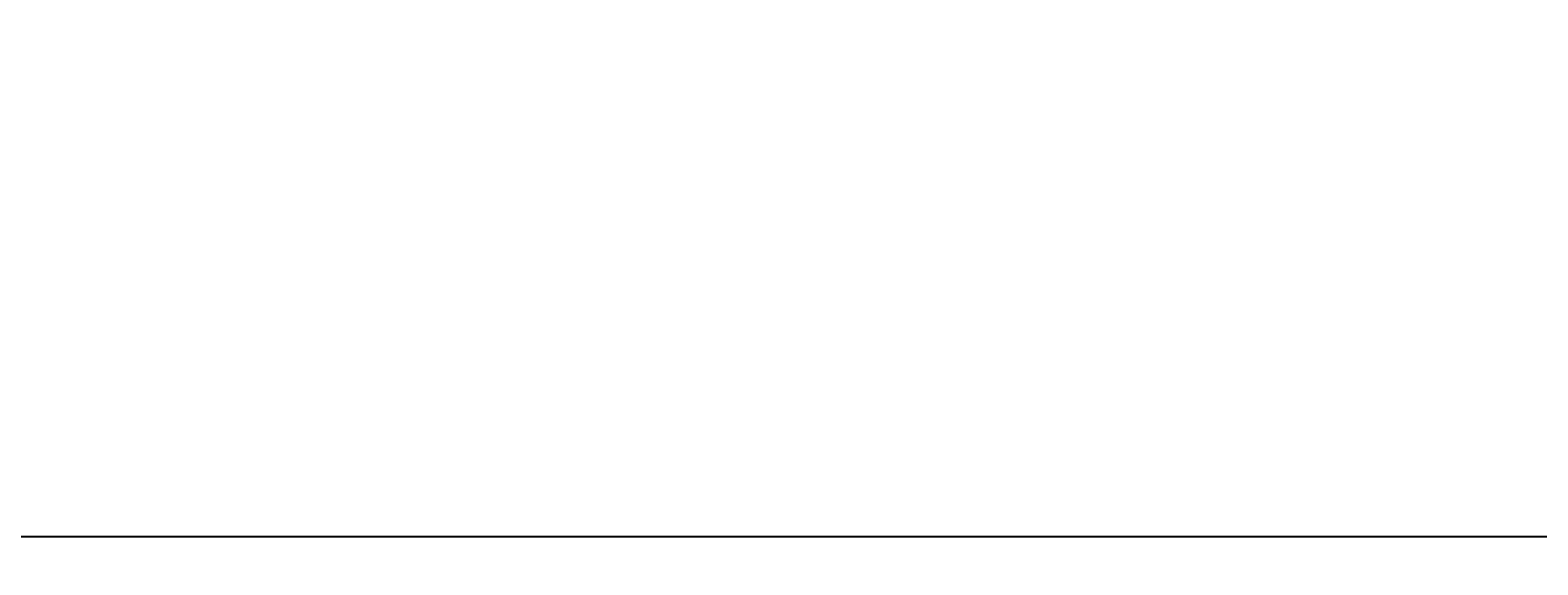
# Model space of a CAD drawing. Units: inches. Extents: x 35362 to 73946, y 43607 to 67532.
# Tile 107 of 134: x 50761 to 50905, y 48917 to 48969. Entities that reach past the tile are written whole.
import ezdxf

# ---------------------------------------------------------------- set-up
doc = ezdxf.new("R2010")
doc.units = ezdxf.units.IN
doc.header["$MEASUREMENT"] = 0
doc.layers.add('A-ANNO-DIMS', color=2, linetype='Continuous', lineweight=18)
doc.styles.get("Standard").update_dxf_attribs({"font": 'arial.ttf'})
doc.dimstyles.get("Standard").update_dxf_attribs({"dimtxt": 0.18, "dimasz": 0.18, "dimexe": 0.18, "dimexo": 0.0625, "dimgap": 0.09, "dimtad": 0, "dimtih": 1, "dimtoh": 1, "dimdec": 4, "dimzin": 0, "dimdsep": 46, "dimtxsty": 'Standard', "dimcen": 0.09, "dimadec": 0, "dimazin": 0, "dimtfac": 1, "dimtdec": 4, "dimtofl": 0, "dimtmove": 0, "dimatfit": 3, "dimfxl": 1, "dimtolj": 1, "dimtzin": 0, "dimarcsym": 0})

# ---------------------------------------------------------------- blocks, each defined once
blk = doc.blocks.new('*D11')
at = {"layer": 'A-ANNO-DIMS', "color": 0, "lineweight": -2, "transparency": 16777216}
for p, q in [((47978.66, 56028.77), (47978.66, 43606.68)), ((53109.76, 56028.77), (53109.76, 43606.68)), ((47978.84, 43606.86), (50543.87, 43606.86)), ((53109.58, 43606.86), (50544.55, 43606.86))]:
    blk.add_line(p, q, dxfattribs=at)
at = {"layer": 'A-ANNO-DIMS', "color": 0, "transparency": 16777216}
for points in [[(47978.84, 43606.89), (47978.84, 43606.83), (47978.66, 43606.86)], [(53109.58, 43606.89), (53109.58, 43606.83), (53109.76, 43606.86)]]:
    blk.add_solid(points, dxfattribs=at)
at = {"layer": 'Defpoints', "color": 0, "transparency": 16777216}
for p in [(47978.66, 56028.84), (53109.76, 56028.84), (53109.76, 43606.86)]:
    blk.add_point(p, dxfattribs=at)
at = {"layer": 'A-ANNO-DIMS', "color": 0, "transparency": 16777216, "insert": (50544.21, 43606.86), "char_height": 0.18, "attachment_point": 5}
blk.add_mtext('\\A1;5131', dxfattribs=at)
blk = doc.blocks.new('*D13')
at = {"layer": 'A-ANNO-DIMS', "color": 0, "lineweight": -2, "transparency": 16777216}
for p, q in [((48373.49, 51694.02), (48373.49, 43606.68)), ((51029.04, 51694.02), (51029.04, 43606.68)), ((48373.67, 43606.86), (49700.8, 43606.86)), ((51028.86, 43606.86), (49701.73, 43606.86))]:
    blk.add_line(p, q, dxfattribs=at)
at = {"layer": 'A-ANNO-DIMS', "color": 0, "transparency": 16777216}
for points in [[(48373.67, 43606.89), (48373.67, 43606.83), (48373.49, 43606.86)], [(51028.86, 43606.89), (51028.86, 43606.83), (51029.04, 43606.86)]]:
    blk.add_solid(points, dxfattribs=at)
at = {"layer": 'Defpoints', "color": 0, "transparency": 16777216}
for p in [(48373.49, 51694.09), (51029.04, 51694.09), (51029.04, 43606.86)]:
    blk.add_point(p, dxfattribs=at)
at = {"layer": 'A-ANNO-DIMS', "color": 0, "transparency": 16777216, "insert": (49701.27, 43606.86), "char_height": 0.18, "attachment_point": 5}
blk.add_mtext('\\A1;2655.6', dxfattribs=at)
blk = doc.blocks.new('*D17')
at = {"layer": 'A-ANNO-DIMS', "color": 0, "lineweight": -2, "transparency": 16777216}
for p, q in [((49923.31, 61293.22), (49923.31, 43606.68)), ((51913.93, 61293.22), (51913.93, 43606.68)), ((49923.49, 43606.86), (50918.16, 43606.86)), ((51913.75, 43606.86), (50919.07, 43606.86))]:
    blk.add_line(p, q, dxfattribs=at)
at = {"layer": 'A-ANNO-DIMS', "color": 0, "transparency": 16777216}
for points in [[(49923.49, 43606.89), (49923.49, 43606.83), (49923.31, 43606.86)], [(51913.75, 43606.89), (51913.75, 43606.83), (51913.93, 43606.86)]]:
    blk.add_solid(points, dxfattribs=at)
at = {"layer": 'Defpoints', "color": 0, "transparency": 16777216}
for p in [(49923.31, 61293.29), (51913.93, 61293.29), (51913.93, 43606.86)]:
    blk.add_point(p, dxfattribs=at)
at = {"layer": 'A-ANNO-DIMS', "color": 0, "transparency": 16777216, "insert": (50918.62, 43606.86), "char_height": 0.18, "attachment_point": 5}
blk.add_mtext('\\A1;1990.6', dxfattribs=at)
blk = doc.blocks.new('*D67')
at = {"layer": 'A-ANNO-DIMS', "color": 0, "lineweight": -2, "transparency": 16777216}
for p, q in [((56873.54, 53351.53), (35361.77, 53351.53)), ((35361.95, 53351.35), (35361.95, 49400.89)), ((35361.95, 45450.07), (35361.95, 49400.53)), ((53793.58, 45449.89), (35361.77, 45449.89))]:
    blk.add_line(p, q, dxfattribs=at)
at = {"layer": 'A-ANNO-DIMS', "color": 0, "transparency": 16777216}
for points in [[(35361.92, 53351.35), (35361.98, 53351.35), (35361.95, 53351.53)], [(35361.92, 45450.07), (35361.98, 45450.07), (35361.95, 45449.89)]]:
    blk.add_solid(points, dxfattribs=at)
at = {"layer": 'Defpoints', "color": 0, "transparency": 16777216}
for p in [(35361.95, 53351.53), (56873.6, 53351.53), (53793.64, 45449.89)]:
    blk.add_point(p, dxfattribs=at)
at = {"layer": 'A-ANNO-DIMS', "color": 0, "transparency": 16777216, "insert": (35361.95, 49400.71), "char_height": 0.18, "attachment_point": 5}
blk.add_mtext('\\A1;7901.6', dxfattribs=at)
blk = doc.blocks.new('*D86')
at = {"layer": 'A-ANNO-DIMS', "color": 0, "lineweight": -2, "transparency": 16777216}
for p, q in [((51285.53, 49320.08), (35361.77, 49320.08)), ((35361.95, 49319.9), (35361.95, 49120.26)), ((35361.95, 48920.26), (35361.95, 49119.9)), ((51285.53, 48920.08), (35361.77, 48920.08))]:
    blk.add_line(p, q, dxfattribs=at)
at = {"layer": 'A-ANNO-DIMS', "color": 0, "transparency": 16777216}
for points in [[(35361.92, 49319.9), (35361.98, 49319.9), (35361.95, 49320.08)], [(35361.92, 48920.26), (35361.98, 48920.26), (35361.95, 48920.08)]]:
    blk.add_solid(points, dxfattribs=at)
at = {"layer": 'Defpoints', "color": 0, "transparency": 16777216}
for p in [(35361.95, 49320.08), (51285.59, 49320.08), (51285.59, 48920.08)]:
    blk.add_point(p, dxfattribs=at)
at = {"layer": 'A-ANNO-DIMS', "color": 0, "transparency": 16777216, "insert": (35361.95, 49120.08), "char_height": 0.18, "attachment_point": 5}
blk.add_mtext('\\A1;400.0', dxfattribs=at)
blk = doc.blocks.new('*D107')
at = {"layer": 'A-ANNO-DIMS', "color": 0, "lineweight": -2, "transparency": 16777216}
for p, q in [((50139.56, 59850.01), (50139.56, 43606.68)), ((51320.81, 59850.01), (51320.81, 43606.68)), ((50139.74, 43606.86), (50729.73, 43606.86)), ((51320.63, 43606.86), (50730.64, 43606.86))]:
    blk.add_line(p, q, dxfattribs=at)
at = {"layer": 'A-ANNO-DIMS', "color": 0, "transparency": 16777216}
for points in [[(50139.74, 43606.89), (50139.74, 43606.83), (50139.56, 43606.86)], [(51320.63, 43606.89), (51320.63, 43606.83), (51320.81, 43606.86)]]:
    blk.add_solid(points, dxfattribs=at)
at = {"layer": 'Defpoints', "color": 0, "transparency": 16777216}
for p in [(50139.56, 59850.08), (51320.81, 59850.08), (51320.81, 43606.86)]:
    blk.add_point(p, dxfattribs=at)
at = {"layer": 'A-ANNO-DIMS', "color": 0, "transparency": 16777216, "insert": (50730.19, 43606.86), "char_height": 0.18, "attachment_point": 5}
blk.add_mtext('\\A1;1181.3', dxfattribs=at)

msp = doc.modelspace()

# ---------------------------------------------------------------- dimensions: what is measured, and where the dimension line sits
at = {"layer": 'A-ANNO-DIMS'}
for base, p1, p2, override, picture, middle in [((51913.931, 43606.859), (49923.307, 61293.286), (51913.931, 61293.286), {"dimdec": 1, "dimlfac": 1, "dimrnd": 0, "dimzin": 0, "dimdsep": 46, "dimlunit": 2}, '*D17', (50918.619, 43606.859)), ((51320.8133, 43606.859), (50139.5627, 59850.0769), (51320.8133, 59850.0769), {"dimdec": 1, "dimlfac": 1, "dimrnd": 0, "dimzin": 0, "dimdsep": 46, "dimlunit": 2}, '*D107', (50730.188, 43606.859)), ((53109.76, 43606.859), (47978.665, 56028.836), (53109.76, 56028.836), {"dimdec": 0, "dimlfac": 1, "dimrnd": 0, "dimzin": 0, "dimdsep": 46, "dimlunit": 2}, '*D11', (50544.212, 43606.859)), ((51029.043, 43606.859), (48373.492, 51694.087), (51029.043, 51694.087), {"dimdec": 1, "dimlfac": 1, "dimrnd": 0, "dimzin": 0, "dimdsep": 46, "dimlunit": 2}, '*D13', (49701.267, 43606.859))]:
    dim = msp.add_linear_dim(base=base, p1=p1, p2=p2, dimstyle='Standard', override=override, dxfattribs=at)
    dim.commit()
    dim.dimension.update_dxf_attribs({"geometry": picture, "text_midpoint": middle})
for base, p1, p2, picture, middle in [((35361.949, 53351.529), (53793.638, 45449.894), (56873.602, 53351.529), '*D67', (35361.949, 49400.712)), ((35361.949, 49320.079), (51285.595, 48920.079), (51285.595, 49320.079), '*D86', (35361.949, 49120.079))]:
    dim = msp.add_linear_dim(base=base, p1=p1, p2=p2, angle=90, dimstyle='Standard', override={"dimdec": 1, "dimlfac": 1, "dimrnd": 0, "dimzin": 0, "dimdsep": 46, "dimlunit": 2}, dxfattribs=at)
    dim.commit()
    dim.dimension.update_dxf_attribs({"geometry": picture, "text_midpoint": middle})

doc.saveas('drawing.dxf')
